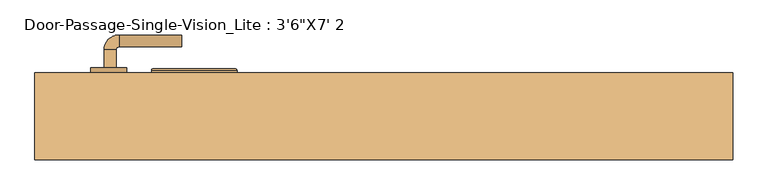
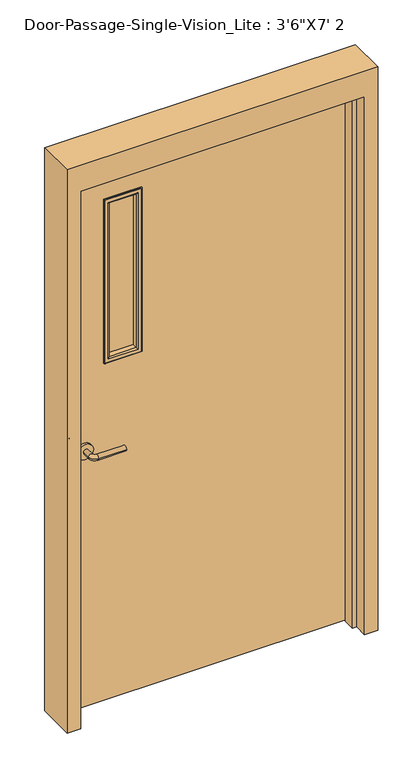
"""IFC4 building model written with IfcOpenShell, lengths in millimetres: door geometry."""

from ifc_helpers import new_model, si_unit, point, frame, frame_2d, origin, place, context, project, spatial, polyline, circle_curve, ellipse_curve, trimmed, segment, composite_curve, outline, extrude, faceted_brep, source, transform, mapped, element, save
from ifc_brep_helpers import plane_surface, cylinder_surface, revolved_surface, advanced_brep


def door_cf1f2706(model_context):
    return source(origin(), model_context, "Body", "SolidModel", [
        advanced_brep(
        [(-468.390625, -14.35, 1016.0), (-448.390625, -14.35, 1016.0), (-448.390625, -44.35, 1016.0), (-468.390625, -44.35, 1016.0), (-443.390625, -49.35, 1016.0), (-443.390625, -69.35, 1016.0), (-338.390625, -69.35, 1016.0), (-338.390625, -49.35, 1016.0)],
        [
            (0, 1, circle_curve(frame((-458.390625, -14.35, 1016.0), z_axis=(0.0, 1.0, 0.0), x_axis=(1.0, 0.0, 0.0)), 10.0)),
            (1, 0, circle_curve(frame((-458.390625, -14.35, 1016.0), z_axis=(0.0, 1.0, 0.0), x_axis=(1.0, 0.0, 0.0)), 10.0)),
            (1, 2),
            (2, 3, circle_curve(frame((-458.390625, -44.35, 1016.0), z_axis=(0.0, 1.0, 0.0), x_axis=(1.0, 0.0, 0.0)), 10.0)),
            (3, 0),
            (3, 2, circle_curve(frame((-458.390625, -44.35, 1016.0), z_axis=(0.0, 1.0, 0.0), x_axis=(1.0, 0.0, 0.0)), 10.0)),
            (4, 5, circle_curve(frame((-443.390625, -59.35, 1016.0), z_axis=(-1.0, 0.0, 0.0), x_axis=(0.0, 1.0, 0.0)), 10.0)),
            (5, 3, circle_curve(frame((-443.390625, -44.35, 1016.0), z_axis=(0.0, 0.0, -1.0), x_axis=(-1.0, 0.0, 0.0)), 25.0)),
            (2, 4, circle_curve(frame((-443.390625, -44.35, 1016.0), z_axis=(0.0, 0.0, 1.0), x_axis=(-1.0, 0.0, 0.0)), 5.0)),
            (5, 4, circle_curve(frame((-443.390625, -59.35, 1016.0), z_axis=(-1.0, 0.0, 0.0), x_axis=(0.0, 1.0, 0.0)), 10.0)),
            (6, 7, circle_curve(frame((-338.390625, -59.35, 1016.0), z_axis=(1.0, 0.0, 0.0), x_axis=(0.0, 1.0, 0.0)), 10.0)),
            (7, 6, circle_curve(frame((-338.390625, -59.35, 1016.0), z_axis=(1.0, 0.0, 0.0), x_axis=(0.0, 1.0, 0.0)), 10.0)),
            (4, 7),
            (6, 5),
        ],
        [
            plane_surface(frame((-458.390625, -14.35, 1016.0), z_axis=(0.0, 1.0, 0.0), x_axis=(0.0, 0.0, 1.0))),
            cylinder_surface(frame((-458.390625, -14.35, 1016.0), z_axis=(0.0, 1.0, 0.0), x_axis=(1.0, 0.0, 0.0)), 10.0),
            revolved_surface(trimmed(ellipse_curve(frame((-458.390625, -44.35, 1016.0), z_axis=(0.0, -1.0, 0.0), x_axis=(1.0, 0.0, 0.0)), 10.0, 10.0), [point((-468.390625, -44.35, 1016.0))], [point((-448.390625, -44.35, 1016.0))], True, "CARTESIAN"), (-443.390625, -44.35, 1016.0), (0.0, 0.0, -1.0)),
            revolved_surface(trimmed(ellipse_curve(frame((-458.390625, -44.35, 1016.0), z_axis=(0.0, -1.0, 0.0), x_axis=(1.0, 0.0, 0.0)), 10.0, 10.0), [point((-448.390625, -44.35, 1016.0))], [point((-468.390625, -44.35, 1016.0))], True, "CARTESIAN"), (-443.390625, -44.35, 1016.0), (0.0, 0.0, -1.0)),
            plane_surface(frame((-338.390625, -59.35, 1016.0), z_axis=(1.0, 0.0, 0.0), x_axis=(0.0, 0.0, 1.0))),
            cylinder_surface(frame((-443.390625, -59.35, 1016.0), z_axis=(-1.0, 0.0, 0.0), x_axis=(0.0, 1.0, 0.0)), 10.0),
        ],
        [
            (0, [[1, 2]]),
            (1, [[3, 4, 5, -2]]),
            (1, [[-5, 6, -3, -1]]),
            (2, [[7, 8, -4, 9]]),
            (3, [[10, -9, -6, -8]]),
            (4, [[11, 12]]),
            (5, [[13, -11, 14, -7]]),
            (5, [[-14, -12, -13, -10]]),
        ],
    ),
        extrude(outline(composite_curve([segment(trimmed(circle_curve(frame_2d((1016.0, -460.890625)), 30.0), [point((1016.0, -490.890625))], [point((1016.0, -430.890625))], False, "CARTESIAN"), True, "CONTINUOUS"), segment(trimmed(circle_curve(frame_2d((1016.0, -460.890625)), 30.0), [point((1016.0, -430.890625))], [point((1016.0, -490.890625))], False, "CARTESIAN"), True, "CONTINUOUS")], self_intersect=False)), frame((0.0, -14.35, 0.0), z_axis=(0.0, 1.0, 0.0), x_axis=(0.0, 0.0, 1.0)), (0.0, 0.0, 1.0), 8.0),
        advanced_brep(
        [(-468.390625, 46.1, 1016.0), (-448.390625, 46.1, 1016.0), (-468.390625, 76.1, 1016.0), (-448.390625, 76.1, 1016.0), (-443.390625, 81.1, 1016.0), (-443.390625, 101.1, 1016.0), (-338.390625, 101.1, 1016.0), (-338.390625, 81.1, 1016.0)],
        [
            (0, 1, circle_curve(frame((-458.390625, 46.1, 1016.0), z_axis=(0.0, -1.0, 0.0), x_axis=(1.0, 0.0, 0.0)), 10.0)),
            (1, 0, circle_curve(frame((-458.390625, 46.1, 1016.0), z_axis=(0.0, -1.0, 0.0), x_axis=(1.0, 0.0, 0.0)), 10.0)),
            (0, 2),
            (2, 3, circle_curve(frame((-458.390625, 76.1, 1016.0), z_axis=(0.0, -1.0, 0.0), x_axis=(1.0, 0.0, 0.0)), 10.0)),
            (3, 1),
            (3, 2, circle_curve(frame((-458.390625, 76.1, 1016.0), z_axis=(0.0, -1.0, 0.0), x_axis=(1.0, 0.0, 0.0)), 10.0)),
            (4, 3, circle_curve(frame((-443.390625, 76.1, 1016.0), z_axis=(0.0, 0.0, 1.0), x_axis=(-1.0, 0.0, 0.0)), 5.0)),
            (2, 5, circle_curve(frame((-443.390625, 76.1, 1016.0), z_axis=(0.0, 0.0, -1.0), x_axis=(-1.0, 0.0, 0.0)), 25.0)),
            (5, 4, circle_curve(frame((-443.390625, 91.1, 1016.0), z_axis=(-1.0, 0.0, 0.0), x_axis=(0.0, -1.0, 0.0)), 10.0)),
            (4, 5, circle_curve(frame((-443.390625, 91.1, 1016.0), z_axis=(-1.0, 0.0, 0.0), x_axis=(0.0, -1.0, 0.0)), 10.0)),
            (6, 7, circle_curve(frame((-338.390625, 91.1, 1016.0), z_axis=(1.0, 0.0, 0.0), x_axis=(0.0, -1.0, 0.0)), 10.0)),
            (7, 6, circle_curve(frame((-338.390625, 91.1, 1016.0), z_axis=(1.0, 0.0, 0.0), x_axis=(0.0, -1.0, 0.0)), 10.0)),
            (5, 6),
            (7, 4),
        ],
        [
            plane_surface(frame((-458.390625, 46.1, 1016.0), z_axis=(0.0, -1.0, 0.0), x_axis=(0.0, 0.0, 1.0))),
            cylinder_surface(frame((-458.390625, 46.1, 1016.0), z_axis=(0.0, -1.0, 0.0), x_axis=(1.0, 0.0, 0.0)), 10.0),
            revolved_surface(trimmed(ellipse_curve(frame((-458.390625, 76.1, 1016.0), z_axis=(0.0, -1.0, 0.0), x_axis=(1.0, 0.0, 0.0)), 10.0, 10.0), [point((-468.390625, 76.1, 1016.0))], [point((-448.390625, 76.1, 1016.0))], True, "CARTESIAN"), (-443.390625, 76.1, 1016.0), (0.0, 0.0, -1.0)),
            revolved_surface(trimmed(ellipse_curve(frame((-458.390625, 76.1, 1016.0), z_axis=(0.0, -1.0, 0.0), x_axis=(1.0, 0.0, 0.0)), 10.0, 10.0), [point((-448.390625, 76.1, 1016.0))], [point((-468.390625, 76.1, 1016.0))], True, "CARTESIAN"), (-443.390625, 76.1, 1016.0), (0.0, 0.0, -1.0)),
            plane_surface(frame((-338.390625, 91.1, 1016.0), z_axis=(1.0, 0.0, 0.0), x_axis=(0.0, 0.0, 1.0))),
            cylinder_surface(frame((-443.390625, 91.1, 1016.0), z_axis=(-1.0, 0.0, 0.0), x_axis=(0.0, -1.0, 0.0)), 10.0),
        ],
        [
            (0, [[1, 2]]),
            (1, [[-1, 3, 4, 5]]),
            (1, [[-2, -5, 6, -3]]),
            (2, [[7, -4, 8, 9]]),
            (3, [[-8, -6, -7, 10]]),
            (4, [[11, 12]]),
            (5, [[-9, 13, -12, 14]]),
            (5, [[-10, -14, -11, -13]]),
        ],
    ),
        extrude(outline(composite_curve([segment(trimmed(circle_curve(frame_2d((1016.0, -460.890625)), 30.0), [point((1016.0, -490.890625))], [point((1016.0, -430.890625))], False, "CARTESIAN"), True, "CONTINUOUS"), segment(trimmed(circle_curve(frame_2d((1016.0, -460.890625)), 30.0), [point((1016.0, -430.890625))], [point((1016.0, -490.890625))], False, "CARTESIAN"), True, "CONTINUOUS")], self_intersect=False)), frame((0.0, 38.1, 0.0), z_axis=(0.0, 1.0, 0.0), x_axis=(0.0, 0.0, 1.0)), (0.0, 0.0, 1.0), 8.0),
        extrude(outline(polyline([(2133.6, -533.4), (0.0, -533.4), (0.0, 533.4), (2133.6, 533.4), (2133.6, -533.4)]), holes=[polyline([(1981.2, -381.0), (1981.2, -254.0), (1346.2, -254.0), (1346.2, -381.0), (1981.2, -381.0)])]), frame((0.0, -6.35, 0.0), z_axis=(0.0, 1.0, 0.0), x_axis=(0.0, 0.0, 1.0)), (0.0, 0.0, 1.0), 44.45),
        faceted_brep([(533.4, -11.1125, 0.0), (533.4, 38.1, 0.0), (584.2, 38.1, 0.0), (584.2, -107.95, 0.0), (533.4, -107.95, 0.0), (533.4, -58.7375, 0.0), (517.525, -58.7375, 0.0), (517.525, -11.1125, 0.0), (533.4, -11.1125, 2133.6), (533.4, 38.1, 2133.6), (-533.4, 38.1, 2133.6), (-533.4, 38.1, 0.0), (-584.2, 38.1, 0.0), (-584.2, 38.1, 2235.2), (584.2, 38.1, 2235.2), (584.2, -107.95, 2235.2), (-584.2, -107.95, 2235.2), (-584.2, -107.95, 0.0), (-533.4, -107.95, 0.0), (-533.4, -107.95, 2133.6), (533.4, -107.95, 2133.6), (533.4, -58.7375, 2133.6), (-533.4, -58.7375, 2133.6), (-533.4, -58.7375, 0.0), (-517.525, -58.7375, 0.0), (-517.525, -58.7375, 2117.725), (517.525, -58.7375, 2117.725), (517.525, -11.1125, 2117.725), (-517.525, -11.1125, 2117.725), (-517.525, -11.1125, 0.0), (-533.4, -11.1125, 0.0), (-533.4, -11.1125, 2133.6)], [[[0, 1, 2, 3, 4, 5, 6, 7]], [[1, 0, 8, 9]], [[2, 1, 9, 10, 11, 12, 13, 14]], [[3, 2, 14, 15]], [[4, 3, 15, 16, 17, 18, 19, 20]], [[5, 4, 20, 21]], [[6, 5, 21, 22, 23, 24, 25, 26]], [[7, 6, 26, 27]], [[0, 7, 27, 28, 29, 30, 31, 8]], [[9, 8, 31, 10]], [[20, 19, 22, 21]], [[26, 25, 28, 27]], [[12, 11, 30, 29, 24, 23, 18, 17]], [[11, 10, 31, 30]], [[13, 12, 17, 16]], [[19, 18, 23, 22]], [[25, 24, 29, 28]], [[15, 14, 13, 16]]]),
        extrude(outline(polyline([(-254.0, 12.7), (-381.0, 12.7), (-381.0, 19.05), (-254.0, 19.05), (-254.0, 12.7)])), frame((0.0, 0.0, 1346.2), z_axis=(0.0, 0.0, 1.0), x_axis=(1.0, 0.0, 0.0)), (0.0, 0.0, 1.0), 635.0),
        advanced_brep(
        [(-381.0, 19.05, 1981.2), (-381.0, 38.1, 1981.2), (-381.0, 38.1, 1346.2), (-381.0, 19.05, 1346.2), (-369.0, 39.1, 1969.2), (-369.0, 19.05, 1969.2), (-369.0, 19.05, 1358.2), (-369.0, 39.1, 1358.2), (-374.0, 44.1, 1974.2), (-374.0, 44.1, 1353.2), (-389.0, 42.1, 1989.2), (-387.0, 44.1, 1987.2), (-387.0, 44.1, 1340.2), (-389.0, 42.1, 1338.2), (-389.0, 38.1, 1989.2), (-389.0, 38.1, 1338.2), (-254.0, 38.1, 1346.2), (-254.0, 19.05, 1346.2), (-266.0, 19.05, 1358.2), (-266.0, 39.1, 1358.2), (-261.0, 44.1, 1353.2), (-248.0, 44.1, 1340.2), (-246.0, 42.1, 1338.2), (-246.0, 38.1, 1338.2), (-254.0, 38.1, 1981.2), (-254.0, 19.05, 1981.2), (-266.0, 19.05, 1969.2), (-266.0, 39.1, 1969.2), (-261.0, 44.1, 1974.2), (-248.0, 44.1, 1987.2), (-246.0, 42.1, 1989.2), (-246.0, 38.1, 1989.2)],
        [
            (0, 1),
            (1, 2),
            (2, 3),
            (3, 0),
            (4, 5),
            (5, 6),
            (6, 7),
            (7, 4),
            (8, 4, ellipse_curve(frame((-374.0, 39.1, 1974.2), z_axis=(-0.7071067811865475, 0.0, -0.7071067811865475), x_axis=(-0.7071067811865474, 0.0, 0.7071067811865476)), 7.0710678, 5.0)),
            (7, 9, ellipse_curve(frame((-374.0, 39.1, 1353.2), z_axis=(-0.7071067811865475, 0.0, 0.7071067811865475), x_axis=(0.7071067811865474, 0.0, 0.7071067811865476)), 7.0710678, 5.0)),
            (9, 8),
            (10, 11, ellipse_curve(frame((-387.0, 42.1, 1987.2), z_axis=(-0.7071067811865475, 0.0, -0.7071067811865475), x_axis=(-0.7071067811865474, 0.0, 0.7071067811865476)), 2.8284271, 2.0)),
            (11, 12),
            (12, 13, ellipse_curve(frame((-387.0, 42.1, 1340.2), z_axis=(-0.7071067811865475, 0.0, 0.7071067811865475), x_axis=(0.7071067811865474, 0.0, 0.7071067811865476)), 2.8284271, 2.0)),
            (13, 10),
            (14, 10),
            (13, 15),
            (15, 14),
            (2, 16),
            (16, 17),
            (17, 3),
            (6, 18),
            (18, 19),
            (19, 7),
            (19, 20, ellipse_curve(frame((-261.0, 39.1, 1353.2), z_axis=(-0.7071067811865475, 0.0, -0.7071067811865475), x_axis=(-0.7071067811865476, 0.0, 0.7071067811865474)), 7.0710678, 5.0)),
            (20, 9),
            (12, 21),
            (21, 22, ellipse_curve(frame((-248.0, 42.1, 1340.2), z_axis=(-0.7071067811865475, 0.0, -0.7071067811865475), x_axis=(-0.7071067811865476, 0.0, 0.7071067811865474)), 2.8284271, 2.0)),
            (22, 13),
            (22, 23),
            (23, 15),
            (16, 24),
            (24, 25),
            (25, 17),
            (18, 26),
            (26, 27),
            (27, 19),
            (27, 28, ellipse_curve(frame((-261.0, 39.1, 1974.2), z_axis=(0.7071067811865475, 0.0, -0.7071067811865475), x_axis=(-0.7071067811865474, 0.0, -0.7071067811865476)), 7.0710678, 5.0)),
            (28, 20),
            (21, 29),
            (29, 30, ellipse_curve(frame((-248.0, 42.1, 1987.2), z_axis=(0.7071067811865475, 0.0, -0.7071067811865475), x_axis=(-0.7071067811865474, 0.0, -0.7071067811865476)), 2.8284271, 2.0)),
            (30, 22),
            (30, 31),
            (31, 23),
            (31, 14),
            (1, 24),
            (0, 25),
            (5, 26),
            (4, 27),
            (8, 28),
            (11, 29),
            (10, 30),
        ],
        [
            plane_surface(frame((-381.0, 38.1, 1981.2), z_axis=(-1.0, 0.0, 0.0), x_axis=(0.0, 0.0, -1.0))),
            plane_surface(frame((-369.0, 19.05, 1969.2), z_axis=(1.0, 0.0, 0.0), x_axis=(0.0, 0.0, -1.0))),
            cylinder_surface(frame((-374.0, 39.1, 1981.2), z_axis=(0.0, 0.0, 1.0), x_axis=(-1.0, 0.0, 0.0)), 5.0),
            cylinder_surface(frame((-387.0, 42.1, 1981.2), z_axis=(0.0, 0.0, 1.0), x_axis=(-1.0, 0.0, 0.0)), 2.0),
            plane_surface(frame((-389.0, 42.1, 1989.2), z_axis=(-1.0, 0.0, 0.0), x_axis=(0.0, 0.0, -1.0))),
            plane_surface(frame((-381.0, 38.1, 1346.2), z_axis=(0.0, 0.0, -1.0), x_axis=(1.0, 0.0, 0.0))),
            plane_surface(frame((-369.0, 19.05, 1358.2), z_axis=(0.0, 0.0, 1.0), x_axis=(1.0, 0.0, 0.0))),
            cylinder_surface(frame((-381.0, 39.1, 1353.2), z_axis=(-1.0, 0.0, 0.0), x_axis=(0.0, 0.0, -1.0)), 5.0),
            cylinder_surface(frame((-381.0, 42.1, 1340.2), z_axis=(-1.0, 0.0, 0.0), x_axis=(0.0, 0.0, -1.0)), 2.0),
            plane_surface(frame((-389.0, 42.1, 1338.2), z_axis=(0.0, 0.0, -1.0), x_axis=(1.0, 0.0, 0.0))),
            plane_surface(frame((-254.0, 38.1, 1346.2), z_axis=(1.0, 0.0, 0.0), x_axis=(0.0, 0.0, 1.0))),
            plane_surface(frame((-266.0, 19.05, 1358.2), z_axis=(-1.0, 0.0, 0.0), x_axis=(0.0, 0.0, 1.0))),
            cylinder_surface(frame((-261.0, 39.1, 1346.2), z_axis=(0.0, 0.0, -1.0), x_axis=(1.0, 0.0, 0.0)), 5.0),
            cylinder_surface(frame((-248.0, 42.1, 1346.2), z_axis=(0.0, 0.0, -1.0), x_axis=(1.0, 0.0, 0.0)), 2.0),
            plane_surface(frame((-246.0, 42.1, 1338.2), z_axis=(1.0, 0.0, 0.0), x_axis=(0.0, 0.0, 1.0))),
            plane_surface(frame((-246.0, 38.1, 1989.2), z_axis=(0.0, -1.0, 0.0), x_axis=(-1.0, 0.0, 0.0))),
            plane_surface(frame((-254.0, 38.1, 1981.2), z_axis=(0.0, 0.0, 1.0), x_axis=(-1.0, 0.0, 0.0))),
            plane_surface(frame((-254.0, 19.05, 1981.2), z_axis=(0.0, -1.0, 0.0), x_axis=(-1.0, 0.0, 0.0))),
            plane_surface(frame((-266.0, 19.05, 1969.2), z_axis=(0.0, 0.0, -1.0), x_axis=(-1.0, 0.0, 0.0))),
            cylinder_surface(frame((-254.0, 39.1, 1974.2), z_axis=(1.0, 0.0, 0.0), x_axis=(0.0, 0.0, 1.0)), 5.0),
            plane_surface(frame((-261.0, 44.1, 1974.2), z_axis=(0.0, 1.0, 0.0), x_axis=(-1.0, 0.0, 0.0))),
            cylinder_surface(frame((-254.0, 42.1, 1987.2), z_axis=(1.0, 0.0, 0.0), x_axis=(0.0, 0.0, 1.0)), 2.0),
            plane_surface(frame((-246.0, 42.1, 1989.2), z_axis=(0.0, 0.0, 1.0), x_axis=(-1.0, 0.0, 0.0))),
        ],
        [
            (0, [[1, 2, 3, 4]]),
            (1, [[5, 6, 7, 8]]),
            (2, [[9, -8, 10, 11]]),
            (3, [[12, 13, 14, 15]]),
            (4, [[16, -15, 17, 18]]),
            (5, [[-3, 19, 20, 21]]),
            (6, [[-7, 22, 23, 24]]),
            (7, [[-10, -24, 25, 26]]),
            (8, [[-14, 27, 28, 29]]),
            (9, [[-17, -29, 30, 31]]),
            (10, [[-20, 32, 33, 34]]),
            (11, [[-23, 35, 36, 37]]),
            (12, [[-25, -37, 38, 39]]),
            (13, [[-28, 40, 41, 42]]),
            (14, [[-30, -42, 43, 44]]),
            (15, [[-31, -44, 45, -18], [46, -32, -19, -2]]),
            (16, [[-33, -46, -1, 47]]),
            (17, [[-21, -34, -47, -4], [48, -35, -22, -6]]),
            (18, [[-36, -48, -5, 49]]),
            (19, [[-38, -49, -9, 50]]),
            (20, [[51, -40, -27, -13], [-26, -39, -50, -11]]),
            (21, [[-41, -51, -12, 52]]),
            (22, [[-43, -52, -16, -45]]),
        ],
    ),
        advanced_brep(
        [(-381.0, 12.7, 1346.2), (-381.0, -6.35, 1346.2), (-381.0, -6.35, 1981.2), (-381.0, 12.7, 1981.2), (-369.0, -7.35, 1358.2), (-369.0, 12.7, 1358.2), (-369.0, 12.7, 1969.2), (-369.0, -7.35, 1969.2), (-374.0, -12.35, 1353.2), (-374.0, -12.35, 1974.2), (-389.0, -10.35, 1338.2), (-387.0, -12.35, 1340.2), (-387.0, -12.35, 1987.2), (-389.0, -10.35, 1989.2), (-389.0, -6.35, 1338.2), (-389.0, -6.35, 1989.2), (-254.0, -6.35, 1981.2), (-254.0, 12.7, 1981.2), (-266.0, 12.7, 1969.2), (-266.0, -7.35, 1969.2), (-261.0, -12.35, 1974.2), (-248.0, -12.35, 1987.2), (-246.0, -10.35, 1989.2), (-246.0, -6.35, 1989.2), (-254.0, -6.35, 1346.2), (-254.0, 12.7, 1346.2), (-266.0, 12.7, 1358.2), (-266.0, -7.35, 1358.2), (-261.0, -12.35, 1353.2), (-248.0, -12.35, 1340.2), (-246.0, -10.35, 1338.2), (-246.0, -6.35, 1338.2)],
        [
            (0, 1),
            (1, 2),
            (2, 3),
            (3, 0),
            (4, 5),
            (5, 6),
            (6, 7),
            (7, 4),
            (8, 4, ellipse_curve(frame((-374.0, -7.35, 1353.2), z_axis=(-0.7071067811865475, 0.0, 0.7071067811865475), x_axis=(-0.7071067811865474, 0.0, -0.7071067811865476)), 7.0710678, 5.0)),
            (7, 9, ellipse_curve(frame((-374.0, -7.35, 1974.2), z_axis=(-0.7071067811865475, 0.0, -0.7071067811865475), x_axis=(0.7071067811865474, 0.0, -0.7071067811865476)), 7.0710678, 5.0)),
            (9, 8),
            (10, 11, ellipse_curve(frame((-387.0, -10.35, 1340.2), z_axis=(-0.7071067811865475, 0.0, 0.7071067811865475), x_axis=(-0.7071067811865474, 0.0, -0.7071067811865476)), 2.8284271, 2.0)),
            (11, 12),
            (12, 13, ellipse_curve(frame((-387.0, -10.35, 1987.2), z_axis=(-0.7071067811865475, 0.0, -0.7071067811865475), x_axis=(0.7071067811865474, 0.0, -0.7071067811865476)), 2.8284271, 2.0)),
            (13, 10),
            (14, 10),
            (13, 15),
            (15, 14),
            (2, 16),
            (16, 17),
            (17, 3),
            (6, 18),
            (18, 19),
            (19, 7),
            (19, 20, ellipse_curve(frame((-261.0, -7.35, 1974.2), z_axis=(-0.7071067811865475, 0.0, 0.7071067811865475), x_axis=(-0.7071067811865476, 0.0, -0.7071067811865474)), 7.0710678, 5.0)),
            (20, 9),
            (12, 21),
            (21, 22, ellipse_curve(frame((-248.0, -10.35, 1987.2), z_axis=(-0.7071067811865475, 0.0, 0.7071067811865475), x_axis=(-0.7071067811865476, 0.0, -0.7071067811865474)), 2.8284271, 2.0)),
            (22, 13),
            (22, 23),
            (23, 15),
            (16, 24),
            (24, 25),
            (25, 17),
            (18, 26),
            (26, 27),
            (27, 19),
            (27, 28, ellipse_curve(frame((-261.0, -7.35, 1353.2), z_axis=(0.7071067811865475, 0.0, 0.7071067811865475), x_axis=(-0.7071067811865474, 0.0, 0.7071067811865476)), 7.0710678, 5.0)),
            (28, 20),
            (21, 29),
            (29, 30, ellipse_curve(frame((-248.0, -10.35, 1340.2), z_axis=(0.7071067811865475, 0.0, 0.7071067811865475), x_axis=(-0.7071067811865474, 0.0, 0.7071067811865476)), 2.8284271, 2.0)),
            (30, 22),
            (30, 31),
            (31, 23),
            (31, 14),
            (1, 24),
            (0, 25),
            (5, 26),
            (4, 27),
            (8, 28),
            (11, 29),
            (10, 30),
        ],
        [
            plane_surface(frame((-381.0, -6.35, 1346.2), z_axis=(-1.0, 0.0, 0.0), x_axis=(0.0, 0.0, 1.0))),
            plane_surface(frame((-369.0, 12.7, 1358.2), z_axis=(1.0, 0.0, 0.0), x_axis=(0.0, 0.0, 1.0))),
            cylinder_surface(frame((-374.0, -7.35, 1346.2), z_axis=(0.0, 0.0, -1.0), x_axis=(-1.0, 0.0, 0.0)), 5.0),
            cylinder_surface(frame((-387.0, -10.35, 1346.2), z_axis=(0.0, 0.0, -1.0), x_axis=(-1.0, 0.0, 0.0)), 2.0),
            plane_surface(frame((-389.0, -10.35, 1338.2), z_axis=(-1.0, 0.0, 0.0), x_axis=(0.0, 0.0, 1.0))),
            plane_surface(frame((-381.0, -6.35, 1981.2), z_axis=(0.0, 0.0, 1.0), x_axis=(1.0, 0.0, 0.0))),
            plane_surface(frame((-369.0, 12.7, 1969.2), z_axis=(0.0, 0.0, -1.0), x_axis=(1.0, 0.0, 0.0))),
            cylinder_surface(frame((-381.0, -7.35, 1974.2), z_axis=(-1.0, 0.0, 0.0), x_axis=(0.0, 0.0, 1.0)), 5.0),
            cylinder_surface(frame((-381.0, -10.35, 1987.2), z_axis=(-1.0, 0.0, 0.0), x_axis=(0.0, 0.0, 1.0)), 2.0),
            plane_surface(frame((-389.0, -10.35, 1989.2), z_axis=(0.0, 0.0, 1.0), x_axis=(1.0, 0.0, 0.0))),
            plane_surface(frame((-254.0, -6.35, 1981.2), z_axis=(1.0, 0.0, 0.0), x_axis=(0.0, 0.0, -1.0))),
            plane_surface(frame((-266.0, 12.7, 1969.2), z_axis=(-1.0, 0.0, 0.0), x_axis=(0.0, 0.0, -1.0))),
            cylinder_surface(frame((-261.0, -7.35, 1981.2), z_axis=(0.0, 0.0, 1.0), x_axis=(1.0, 0.0, 0.0)), 5.0),
            cylinder_surface(frame((-248.0, -10.35, 1981.2), z_axis=(0.0, 0.0, 1.0), x_axis=(1.0, 0.0, 0.0)), 2.0),
            plane_surface(frame((-246.0, -10.35, 1989.2), z_axis=(1.0, 0.0, 0.0), x_axis=(0.0, 0.0, -1.0))),
            plane_surface(frame((-246.0, -6.35, 1338.2), z_axis=(0.0, 1.0, 0.0), x_axis=(-1.0, 0.0, 0.0))),
            plane_surface(frame((-254.0, -6.35, 1346.2), z_axis=(0.0, 0.0, -1.0), x_axis=(-1.0, 0.0, 0.0))),
            plane_surface(frame((-254.0, 12.7, 1346.2), z_axis=(0.0, 1.0, 0.0), x_axis=(-1.0, 0.0, 0.0))),
            plane_surface(frame((-266.0, 12.7, 1358.2), z_axis=(0.0, 0.0, 1.0), x_axis=(-1.0, 0.0, 0.0))),
            cylinder_surface(frame((-254.0, -7.35, 1353.2), z_axis=(1.0, 0.0, 0.0), x_axis=(0.0, 0.0, -1.0)), 5.0),
            plane_surface(frame((-261.0, -12.35, 1353.2), z_axis=(0.0, -1.0, 0.0), x_axis=(-1.0, 0.0, 0.0))),
            cylinder_surface(frame((-254.0, -10.35, 1340.2), z_axis=(1.0, 0.0, 0.0), x_axis=(0.0, 0.0, -1.0)), 2.0),
            plane_surface(frame((-246.0, -10.35, 1338.2), z_axis=(0.0, 0.0, -1.0), x_axis=(-1.0, 0.0, 0.0))),
        ],
        [
            (0, [[1, 2, 3, 4]]),
            (1, [[5, 6, 7, 8]]),
            (2, [[9, -8, 10, 11]]),
            (3, [[12, 13, 14, 15]]),
            (4, [[16, -15, 17, 18]]),
            (5, [[-3, 19, 20, 21]]),
            (6, [[-7, 22, 23, 24]]),
            (7, [[-10, -24, 25, 26]]),
            (8, [[-14, 27, 28, 29]]),
            (9, [[-17, -29, 30, 31]]),
            (10, [[-20, 32, 33, 34]]),
            (11, [[-23, 35, 36, 37]]),
            (12, [[-25, -37, 38, 39]]),
            (13, [[-28, 40, 41, 42]]),
            (14, [[-30, -42, 43, 44]]),
            (15, [[-31, -44, 45, -18], [46, -32, -19, -2]]),
            (16, [[-33, -46, -1, 47]]),
            (17, [[-21, -34, -47, -4], [48, -35, -22, -6]]),
            (18, [[-36, -48, -5, 49]]),
            (19, [[-38, -49, -9, 50]]),
            (20, [[51, -40, -27, -13], [-26, -39, -50, -11]]),
            (21, [[-41, -51, -12, 52]]),
            (22, [[-43, -52, -16, -45]]),
        ],
    ),
    ])


if __name__ == "__main__":
    model = new_model("IFC4")
    model_context = context("Model", 3, world=origin())
    ifc_project = project(units=[si_unit("LENGTHUNIT", "METRE", prefix="MILLI")], contexts=[model_context])
    site = spatial("IfcSite", under=ifc_project)
    building = spatial("IfcBuilding", under=site)
    placement = place(None, origin())
    door_shape = door_cf1f2706(model_context)
    element("IfcDoor", 1, ObjectType="Door-Passage-Single-Vision_Lite : 3'6\"X7' 2", at=placement, inside=building, context=model_context, shape_type="MappedRepresentation", body=[
        mapped(door_shape, transform((0.0, 0.0, 0.0), x_axis=(1.0, 0.0, 0.0), y_axis=(0.0, 1.0, 0.0), z_axis=(0.0, 0.0, 1.0))),
    ])
    save(model, "model.ifc")

# Revit data of these elements
# Type "Door-Passage-Single-Vision_Lite : 3'6\"X7' 2"
#   Type Mark = "14"
#   Assembly Code = "B2030100"
#   Analytic Construction = "Wooden"
#   Thickness = 0' - 1 3/4"
#   Thermal Resistance (R) = 2.5876 (h·ft²·°F)/BTU
#   Swing Angle [instance default] = 90.00°
#   Strike Height = 3' - 4"
#   Rough Width [instance default] = 3' - 10"
#   Rough Height [instance default] = 7' - 4"
#   MFOpeningHeight [instance default] = 0' - 4"
#   MFOpeningWidth [instance default] = 0' - 4"
#   Inset Calculate [instance default] = 0' - 4"
#   Masonry Inset [instance default] = 0' - 1"
#   Height = 7' - 0"
#   Width = 3' - 6"
#   Heat Transfer Coefficient (U) = 0.3865 BTU/(h·ft²·°F)
#   Masonry Frame Depth = 0' - 5 3/4"
#   Masonry Frame [instance default] = yes
#   Function = 1
#   Dry Wall Frame [instance default] = no
#   Panel Material = Wood - Birch
#   Glazing = Glass
#   Glass Stop Material = Metal - Paint Finish - Grey
#   Frame Material = Metal - Paint Finish - Grey
#   Door Handle Material = Aluminum
#   Visual Light Transmittance = 0
#   Solar Heat Gain Coefficient = 0
#   Wall Closure = (empty or 0)
# Element 1 (IfcDoor, "Door-Passage-Single-Vision_Lite : 3'6\"X7' 2")
#   Materials on its faces: "Metal - Paint Finish - Grey", "Aluminum", "Wood - Birch", "Glass"
# Materials
#   "Wood - Birch": class "Wood", colour RGB 166 116 52, transparency 0, Cost = 0
#   "Glass": class "Glass", colour RGB 0 128 192, transparency 0.75, Description = "Soda Lime Glass", Cost = 0
#   "Metal - Paint Finish - Grey": class "Paint", colour RGB 104 104 104, transparency 0, Cost = 0
#   "Aluminum": class "Metal", colour RGB 247 247 247, transparency 0, Description = "Aluminum 6061", Cost = 0
